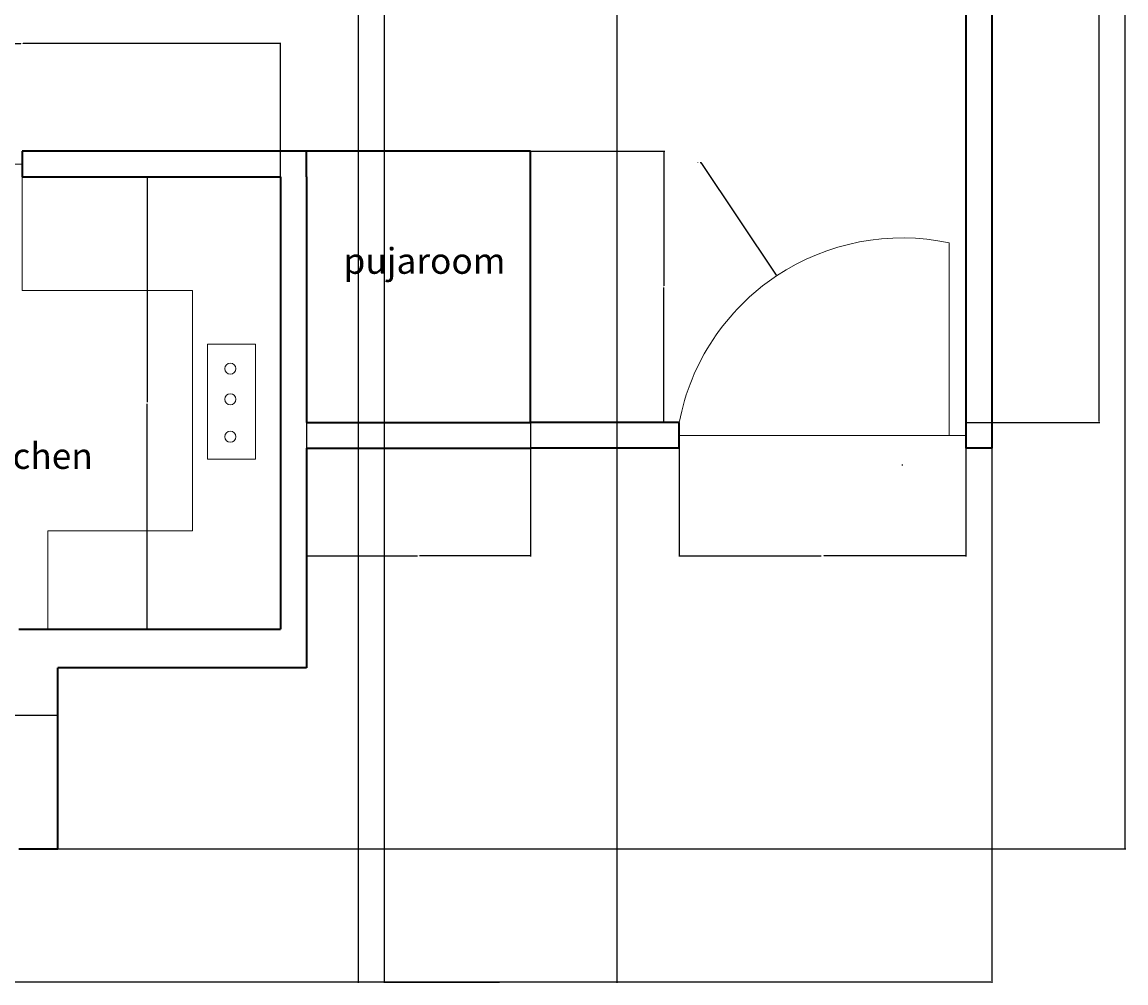
# Model space of a CAD drawing. Units: inches. Extents: x 177 to 785, y -381 to 206.
# Tile 4 of 5: x 529 to 785, y -381 to -158. Entities that reach past the tile are written whole.
import ezdxf

# ---------------------------------------------------------------- set-up
doc = ezdxf.new("R2010")
doc.units = ezdxf.units.IN
doc.header["$MEASUREMENT"] = 0
for name, color, linetype, lineweight in [('A-ANNO-DIMS', 2, 'Continuous', 18), ('A-AREA-IDEN', 7, 'Continuous', 20), ('A-DOOR', 4, 'Continuous', 18), ('A-FLOR-CASE', 9, 'Continuous', 20), ('A-WALL', 7, 'Continuous', 35), ('equipments', 2, 'Continuous', 18)]:
    doc.layers.add(name, color=color, linetype=linetype, lineweight=lineweight)
doc.styles.get("Standard").update_dxf_attribs({"font": 'arial.ttf'})
doc.dimstyles.get("Standard").update_dxf_attribs({"dimtxt": 0.18, "dimasz": 0.18, "dimexe": 0.18, "dimexo": 0.0625, "dimgap": 0.09, "dimtad": 0, "dimtih": 1, "dimtoh": 1, "dimdec": 4, "dimzin": 0, "dimdsep": 46, "dimtxsty": 'Standard', "dimcen": 0.09, "dimadec": 0, "dimazin": 0, "dimtfac": 1, "dimtdec": 4, "dimtofl": 0, "dimtmove": 0, "dimatfit": 3, "dimfxl": 1, "dimtolj": 1, "dimtzin": 0, "dimarcsym": 0})

# ---------------------------------------------------------------- blocks, each defined once
blk = doc.blocks.new('*D23')
at = {"layer": 'A-ANNO-DIMS', "color": 0, "lineweight": -2, "transparency": 16777216}
for p, q in [((754.33, -257.2), (754.33, -381.27)), ((202.33, -275.2), (202.33, -381.27)), ((202.51, -381.09), (478.04, -381.09)), ((754.15, -381.09), (478.62, -381.09))]:
    blk.add_line(p, q, dxfattribs=at)
at = {"layer": 'A-ANNO-DIMS', "color": 0, "transparency": 16777216}
for points in [[(202.51, -381.06), (202.51, -381.12), (202.33, -381.09)], [(754.15, -381.06), (754.15, -381.12), (754.33, -381.09)]]:
    blk.add_solid(points, dxfattribs=at)
at = {"layer": 'Defpoints', "color": 0, "transparency": 16777216}
for p in [(754.33, -257.14), (202.33, -275.14), (754.33, -381.09)]:
    blk.add_point(p, dxfattribs=at)
at = {"layer": 'A-ANNO-DIMS', "color": 0, "transparency": 16777216, "insert": (478.33, -381.09), "char_height": 0.18, "attachment_point": 5}
blk.add_mtext('\\A1;552', dxfattribs=at)
blk = doc.blocks.new('*D24')
at = {"layer": 'A-ANNO-DIMS', "color": 0, "lineweight": -2, "transparency": 16777216}
for p, q in [((610.39, 174.86), (785.46, 174.86)), ((785.28, 174.68), (785.28, -87.46)), ((785.28, -349.96), (785.28, -87.82)), ((537.67, -350.14), (785.46, -350.14))]:
    blk.add_line(p, q, dxfattribs=at)
at = {"layer": 'A-ANNO-DIMS', "color": 0, "transparency": 16777216}
for points in [[(785.25, 174.68), (785.31, 174.68), (785.28, 174.86)], [(785.25, -349.96), (785.31, -349.96), (785.28, -350.14)]]:
    blk.add_solid(points, dxfattribs=at)
at = {"layer": 'Defpoints', "color": 0, "transparency": 16777216}
for p in [(610.33, 174.86), (537.61, -350.14), (785.28, -350.14)]:
    blk.add_point(p, dxfattribs=at)
at = {"layer": 'A-ANNO-DIMS', "color": 0, "transparency": 16777216, "insert": (785.28, -87.64), "char_height": 0.18, "attachment_point": 5}
blk.add_mtext('\\A1;525', dxfattribs=at)
blk = doc.blocks.new('*D33')
at = {"layer": 'A-ANNO-DIMS', "color": 0, "lineweight": -2, "transparency": 16777216}
for p, q in [((607.33, -68.2), (607.33, -381.27)), ((439.33, -74.2), (439.33, -381.27)), ((439.51, -381.09), (523.05, -381.09)), ((607.15, -381.09), (523.61, -381.09))]:
    blk.add_line(p, q, dxfattribs=at)
at = {"layer": 'A-ANNO-DIMS', "color": 0, "transparency": 16777216}
for points in [[(439.51, -381.06), (439.51, -381.12), (439.33, -381.09)], [(607.15, -381.06), (607.15, -381.12), (607.33, -381.09)]]:
    blk.add_solid(points, dxfattribs=at)
at = {"layer": 'Defpoints', "color": 0, "transparency": 16777216}
for p in [(607.33, -68.14), (439.33, -74.14), (607.33, -381.09)]:
    blk.add_point(p, dxfattribs=at)
at = {"layer": 'A-ANNO-DIMS', "color": 0, "transparency": 16777216, "insert": (523.33, -381.09), "char_height": 0.18, "attachment_point": 5}
blk.add_mtext('\\A1;168', dxfattribs=at)
blk = doc.blocks.new('*D40')
at = {"layer": 'A-ANNO-DIMS', "color": 0, "lineweight": -2, "transparency": 16777216}
for p, q in [((613.33, -29.2), (613.33, -381.27)), ((667.33, -29.2), (667.33, -381.27)), ((613.51, -381.09), (640.11, -381.09)), ((667.15, -381.09), (640.55, -381.09))]:
    blk.add_line(p, q, dxfattribs=at)
at = {"layer": 'A-ANNO-DIMS', "color": 0, "transparency": 16777216}
for points in [[(613.51, -381.06), (613.51, -381.12), (613.33, -381.09)], [(667.15, -381.06), (667.15, -381.12), (667.33, -381.09)]]:
    blk.add_solid(points, dxfattribs=at)
at = {"layer": 'Defpoints', "color": 0, "transparency": 16777216}
for p in [(613.33, -29.14), (667.33, -29.14), (667.33, -381.09)]:
    blk.add_point(p, dxfattribs=at)
at = {"layer": 'A-ANNO-DIMS', "color": 0, "transparency": 16777216, "insert": (640.33, -381.09), "char_height": 0.18, "attachment_point": 5}
blk.add_mtext('\\A1;54', dxfattribs=at)
blk = doc.blocks.new('*D49')
at = {"layer": 'A-ANNO-DIMS', "color": 0, "lineweight": -2, "transparency": 16777216}
for p, q in [((469.33, -194.08), (469.33, -163.01)), ((469.51, -163.19), (529.05, -163.19)), ((589.15, -163.19), (529.61, -163.19)), ((589.33, -194.08), (589.33, -163.01))]:
    blk.add_line(p, q, dxfattribs=at)
at = {"layer": 'A-ANNO-DIMS', "color": 0, "transparency": 16777216}
for points in [[(469.51, -163.16), (469.51, -163.22), (469.33, -163.19)], [(589.15, -163.16), (589.15, -163.22), (589.33, -163.19)]]:
    blk.add_solid(points, dxfattribs=at)
at = {"layer": 'Defpoints', "color": 0, "transparency": 16777216}
for p in [(589.33, -163.19), (469.33, -194.14), (589.33, -194.14)]:
    blk.add_point(p, dxfattribs=at)
at = {"layer": 'A-ANNO-DIMS', "color": 0, "transparency": 16777216, "insert": (529.33, -163.19), "char_height": 0.18, "attachment_point": 5}
blk.add_mtext('\\A1;120', dxfattribs=at)
blk = doc.blocks.new('*D50')
at = {"layer": 'A-ANNO-DIMS', "color": 0, "lineweight": -2, "transparency": 16777216}
for p, q in [((589.27, -194.14), (558.2, -194.14)), ((558.38, -194.32), (558.38, -246.46)), ((558.38, -298.96), (558.38, -246.82)), ((589.27, -299.14), (558.2, -299.14))]:
    blk.add_line(p, q, dxfattribs=at)
at = {"layer": 'A-ANNO-DIMS', "color": 0, "transparency": 16777216}
for points in [[(558.35, -194.32), (558.41, -194.32), (558.38, -194.14)], [(558.35, -298.96), (558.41, -298.96), (558.38, -299.14)]]:
    blk.add_solid(points, dxfattribs=at)
at = {"layer": 'Defpoints', "color": 0, "transparency": 16777216}
for p in [(558.38, -194.14), (589.33, -194.14), (589.33, -299.14)]:
    blk.add_point(p, dxfattribs=at)
at = {"layer": 'A-ANNO-DIMS', "color": 0, "transparency": 16777216, "insert": (558.38, -246.64), "char_height": 0.18, "attachment_point": 5}
blk.add_mtext('\\A1;105', dxfattribs=at)
blk = doc.blocks.new('*D51')
at = {"layer": 'A-ANNO-DIMS', "color": 0, "lineweight": -2, "transparency": 16777216}
for p, q in [((595.33, -251.2), (595.33, -282.27)), ((647.33, -251.2), (647.33, -282.27)), ((595.51, -282.09), (621.11, -282.09)), ((647.15, -282.09), (621.55, -282.09))]:
    blk.add_line(p, q, dxfattribs=at)
at = {"layer": 'A-ANNO-DIMS', "color": 0, "transparency": 16777216}
for points in [[(595.51, -282.06), (595.51, -282.12), (595.33, -282.09)], [(647.15, -282.06), (647.15, -282.12), (647.33, -282.09)]]:
    blk.add_solid(points, dxfattribs=at)
at = {"layer": 'Defpoints', "color": 0, "transparency": 16777216}
for p in [(595.33, -251.14), (647.33, -251.14), (595.33, -282.09)]:
    blk.add_point(p, dxfattribs=at)
at = {"layer": 'A-ANNO-DIMS', "color": 0, "transparency": 16777216, "insert": (621.33, -282.09), "char_height": 0.18, "attachment_point": 5}
blk.add_mtext('\\A1;52', dxfattribs=at)
blk = doc.blocks.new('*D52')
at = {"layer": 'A-ANNO-DIMS', "color": 0, "lineweight": -2, "transparency": 16777216}
for p, q in [((647.39, -188.14), (678.46, -188.14)), ((678.28, -188.32), (678.28, -219.46)), ((678.28, -250.96), (678.28, -219.82)), ((647.39, -251.14), (678.46, -251.14))]:
    blk.add_line(p, q, dxfattribs=at)
at = {"layer": 'A-ANNO-DIMS', "color": 0, "transparency": 16777216}
for points in [[(678.25, -188.32), (678.31, -188.32), (678.28, -188.14)], [(678.25, -250.96), (678.31, -250.96), (678.28, -251.14)]]:
    blk.add_solid(points, dxfattribs=at)
at = {"layer": 'Defpoints', "color": 0, "transparency": 16777216}
for p in [(647.33, -188.14), (647.33, -251.14), (678.28, -251.14)]:
    blk.add_point(p, dxfattribs=at)
at = {"layer": 'A-ANNO-DIMS', "color": 0, "transparency": 16777216, "insert": (678.28, -219.64), "char_height": 0.18, "attachment_point": 5}
blk.add_mtext('\\A1;63', dxfattribs=at)
blk = doc.blocks.new('*D53')
at = {"layer": 'A-ANNO-DIMS', "color": 0, "lineweight": -2, "transparency": 16777216}
for p, q in [((748.39, -35.14), (779.46, -35.14)), ((779.28, -35.32), (779.28, -142.96)), ((779.28, -250.96), (779.28, -143.32)), ((748.39, -251.14), (779.46, -251.14))]:
    blk.add_line(p, q, dxfattribs=at)
at = {"layer": 'A-ANNO-DIMS', "color": 0, "transparency": 16777216}
for points in [[(779.25, -35.32), (779.31, -35.32), (779.28, -35.14)], [(779.25, -250.96), (779.31, -250.96), (779.28, -251.14)]]:
    blk.add_solid(points, dxfattribs=at)
at = {"layer": 'Defpoints', "color": 0, "transparency": 16777216}
for p in [(748.33, -35.14), (748.33, -251.14), (779.28, -251.14)]:
    blk.add_point(p, dxfattribs=at)
at = {"layer": 'A-ANNO-DIMS', "color": 0, "transparency": 16777216, "insert": (779.28, -143.14), "char_height": 0.18, "attachment_point": 5}
blk.add_mtext('\\A1;216', dxfattribs=at)
blk = doc.blocks.new('*D55')
at = {"layer": 'A-ANNO-DIMS', "color": 0, "lineweight": -2, "transparency": 16777216}
for p, q in [((681.83, -251.2), (681.83, -282.27)), ((748.33, -251.2), (748.33, -282.27)), ((682.01, -282.09), (714.76, -282.09)), ((748.15, -282.09), (715.41, -282.09))]:
    blk.add_line(p, q, dxfattribs=at)
at = {"layer": 'A-ANNO-DIMS', "color": 0, "transparency": 16777216}
for points in [[(682.01, -282.06), (682.01, -282.12), (681.83, -282.09)], [(748.15, -282.06), (748.15, -282.12), (748.33, -282.09)]]:
    blk.add_solid(points, dxfattribs=at)
at = {"layer": 'Defpoints', "color": 0, "transparency": 16777216}
for p in [(681.83, -251.14), (748.33, -251.14), (681.83, -282.09)]:
    blk.add_point(p, dxfattribs=at)
at = {"layer": 'A-ANNO-DIMS', "color": 0, "transparency": 16777216, "insert": (715.08, -282.09), "char_height": 0.18, "attachment_point": 5}
blk.add_mtext('\\A1;66.5', dxfattribs=at)
blk = doc.blocks.new('*D57')
at = {"layer": 'A-ANNO-DIMS', "color": 0, "lineweight": -2, "transparency": 16777216}
for p, q in [((426.79, -350.08), (426.79, -319.01)), ((426.97, -319.19), (481.74, -319.19)), ((537.43, -319.19), (482.65, -319.19)), ((537.61, -350.08), (537.61, -319.01))]:
    blk.add_line(p, q, dxfattribs=at)
at = {"layer": 'A-ANNO-DIMS', "color": 0, "transparency": 16777216}
for points in [[(426.97, -319.16), (426.97, -319.22), (426.79, -319.19)], [(537.43, -319.16), (537.43, -319.22), (537.61, -319.19)]]:
    blk.add_solid(points, dxfattribs=at)
at = {"layer": 'Defpoints', "color": 0, "transparency": 16777216}
for p in [(537.61, -319.19), (426.79, -350.14), (537.61, -350.14)]:
    blk.add_point(p, dxfattribs=at)
at = {"layer": 'A-ANNO-DIMS', "color": 0, "transparency": 16777216, "insert": (482.2, -319.19), "char_height": 0.18, "attachment_point": 5}
blk.add_mtext('\\A1;110.82', dxfattribs=at)
blk = doc.blocks.new('*D75')
at = {"layer": 'A-ANNO-DIMS', "color": 0, "lineweight": -2, "transparency": 16777216}
for p, q in [((686.68, -190.82), (686.86, -190.82)), ((686.86, -190.82), (704.29, -216.98)), ((733.51, -260.99), (733.69, -260.99)), ((733.6, -261.08), (733.6, -260.9))]:
    blk.add_line(p, q, dxfattribs=at)
at = {"layer": 'A-ANNO-DIMS', "color": 0, "transparency": 16777216}
blk.add_solid([(704.31, -216.97), (704.26, -217), (704.39, -217.13)], dxfattribs=at)
at = {"layer": 'Defpoints', "color": 0, "transparency": 16777216}
for p in [(704.39, -217.13), (733.6, -260.99)]:
    blk.add_point(p, dxfattribs=at)
at = {"layer": 'A-ANNO-DIMS', "color": 0, "transparency": 16777216, "insert": (686.27, -190.82), "char_height": 0.18, "attachment_point": 5}
blk.add_mtext('\\A1;R52.7', dxfattribs=at)

msp = doc.modelspace()

# ---------------------------------------------------------------- linework, layer by layer
at = {"layer": 'A-DOOR'}
for p, q in [((499.3284, -191.1401), (529.3284, -191.1401)), ((744.4598, -254.1401), (744.4598, -209.4242)), ((681.8328, -254.1401), (748.3284, -254.1401)), ((748.3284, -254.1401), (744.4598, -254.1401))]:
    msp.add_line(p, q, dxfattribs=at)
msp.add_arc((733.6032, -260.9936), 52.6998, 78.11151, 169.223692, dxfattribs=at)
at = {"layer": 'A-FLOR-CASE'}
for p, q in [((529.3284, -194.1401), (529.3284, -220.4869)), ((529.3284, -220.4869), (568.8441, -220.4869)), ((568.8441, -220.4869), (568.8441, -276.3183)), ((568.8441, -276.3183), (535.3205, -276.3183)), ((535.3205, -276.3183), (535.3205, -299.1401))]:
    msp.add_line(p, q, dxfattribs=at)
at = {"layer": 'A-WALL'}
for p, q in [((748.3284, -35.1401), (748.3284, -251.1401)), ((754.3284, -35.1401), (754.3284, -257.1401)), ((589.3284, -188.1401), (529.3284, -188.1401)), ((529.3284, -188.1401), (529.3284, -191.1401)), ((595.3284, -188.1401), (589.3284, -188.1401)), ((595.3284, -194.1401), (595.3284, -188.1401)), ((647.3284, -188.1401), (595.3284, -188.1401)), ((647.3284, -197.1401), (647.3284, -188.1401)), ((529.3284, -191.1401), (529.3284, -194.1401)), ((529.3284, -194.1401), (589.3284, -194.1401)), ((589.3284, -194.1401), (589.3284, -299.1401)), ((595.3284, -194.1401), (595.3284, -251.1401)), ((647.3284, -251.1401), (647.3284, -197.1401)), ((595.3284, -251.1401), (647.3284, -251.1401)), ((681.8328, -251.1401), (647.3284, -251.1401)), ((681.8328, -257.1401), (681.8328, -251.1401)), ((748.3284, -251.1401), (748.3284, -257.1401)), ((595.3284, -257.1401), (647.3284, -257.1401)), ((595.3284, -257.1401), (595.3284, -308.1401)), ((681.8328, -257.1401), (647.3284, -257.1401)), ((754.3284, -257.1401), (748.3284, -257.1401)), ((528.6096, -299.1401), (589.3284, -299.1401)), ((589.3284, -308.1401), (537.6096, -308.1401)), ((537.6096, -350.1401), (537.6096, -308.1401)), ((595.3284, -308.1401), (589.3284, -308.1401)), ((528.6096, -350.1401), (537.6096, -350.1401))]:
    msp.add_line(p, q, dxfattribs=at)
at = {"layer": 'equipments'}
msp.add_lwpolyline([(572.3294, -233.0046), (583.4713, -233.0046), (583.4713, -259.6285), (572.3294, -259.6285)], close=True, dxfattribs=at)
for centre in [(577.6581, -238.6521), (577.6581, -245.7518), (577.6581, -254.465)]:
    msp.add_circle(centre, 1.2909, dxfattribs=at)

# ---------------------------------------------------------------- texts
at = {"layer": 'A-AREA-IDEN', "char_height": 6, "attachment_point": 1}
for s, insert in [('pujaroom', (603.9192, -210.633)), ('kitchen', (517.2216, -255.9235))]:
    msp.add_mtext_dynamic_manual_height_columns(s, width=20.406791, gutter_width=1, heights=[0], dxfattribs=dict(at, insert=insert))

# ---------------------------------------------------------------- dimensions: what is measured, and where the dimension line sits
at = {"layer": 'A-ANNO-DIMS'}
for base, p1, p2, angle, override, picture, middle in [((785.2784, -350.1401), (610.3284, 174.8599), (537.6096, -350.1401), 90, {"dimdec": 0, "dimlfac": 1, "dimrnd": 0, "dimzin": 0, "dimdsep": 46, "dimlunit": 2}, '*D24', (785.2784, -87.6401)), ((779.2784, -251.1401), (748.3284, -35.1401), (748.3284, -251.1401), 270, {"dimdec": 0, "dimlfac": 1, "dimrnd": 0, "dimzin": 0, "dimdsep": 46, "dimlunit": 2}, '*D53', (779.2784, -143.1401)), ((678.2784, -251.1401), (647.3284, -188.1401), (647.3284, -251.1401), 270, {"dimdec": 0, "dimlfac": 1, "dimrnd": 0, "dimzin": 0, "dimdsep": 46, "dimlunit": 2}, '*D52', (678.2784, -219.6401)), ((558.3784, -194.1401), (589.3284, -299.1401), (589.3284, -194.1401), 90, {"dimdec": 0, "dimlfac": 1, "dimrnd": 0, "dimzin": 0, "dimdsep": 46, "dimlunit": 2}, '*D50', (558.3784, -246.6401)), ((595.3284, -282.0901), (647.3284, -251.1401), (595.3284, -251.1401), 180, {"dimdec": 0, "dimlfac": 1, "dimrnd": 0, "dimzin": 0, "dimdsep": 46, "dimlunit": 2}, '*D51', (621.3284, -282.0901)), ((681.8328, -282.0901), (748.3284, -251.1401), (681.8328, -251.1401), 180, {"dimdec": 1, "dimlfac": 1, "dimrnd": 0, "dimzin": 0, "dimdsep": 46, "dimlunit": 2}, '*D55', (715.0806, -282.0901))]:
    dim = msp.add_linear_dim(base=base, p1=p1, p2=p2, angle=angle, dimstyle='Standard', override=override, dxfattribs=at)
    dim.commit()
    dim.dimension.update_dxf_attribs({"geometry": picture, "text_midpoint": middle})
for base, p1, p2, override, picture, middle in [((667.3284, -381.0901), (613.3284, -29.1401), (667.3284, -29.1401), {"dimdec": 0, "dimlfac": 1, "dimrnd": 0, "dimzin": 0, "dimdsep": 46, "dimlunit": 2}, '*D40', (640.3284, -381.0901)), ((607.3284, -381.0901), (439.3284, -74.1401), (607.3284, -68.1401), {"dimdec": 0, "dimlfac": 1, "dimrnd": 0, "dimzin": 0, "dimdsep": 46, "dimlunit": 2}, '*D33', (523.3284, -381.0901)), ((589.3284, -163.1901), (469.3284, -194.1401), (589.3284, -194.1401), {"dimdec": 0, "dimlfac": 1, "dimrnd": 0, "dimzin": 0, "dimdsep": 46, "dimlunit": 2}, '*D49', (529.3284, -163.1901)), ((754.3284, -381.0901), (202.3284, -275.1401), (754.3284, -257.1401), {"dimdec": 0, "dimlfac": 1, "dimrnd": 0, "dimzin": 0, "dimdsep": 46, "dimlunit": 2}, '*D23', (478.3284, -381.0901)), ((537.6096, -319.1901), (426.7874, -350.1401), (537.6096, -350.1401), {"dimdec": 2, "dimlfac": 1, "dimrnd": 0, "dimzin": 0, "dimdsep": 46, "dimlunit": 2}, '*D57', (482.1985, -319.1901))]:
    dim = msp.add_linear_dim(base=base, p1=p1, p2=p2, dimstyle='Standard', override=override, dxfattribs=at)
    dim.commit()
    dim.dimension.update_dxf_attribs({"geometry": picture, "text_midpoint": middle})
dim = msp.add_radius_dim(center=(733.6032, -260.9936), mpoint=(704.3881, -217.1331), dimstyle='Standard', override={"dimdec": 1, "dimlfac": 1, "dimrnd": 0, "dimzin": 0, "dimdsep": 46, "dimlunit": 2}, dxfattribs=at)
dim.commit()
dim.dimension.update_dxf_attribs({"geometry": '*D75', "text_midpoint": (686.2691, -190.8168), "dimtype": 164})

doc.saveas('drawing.dxf')
